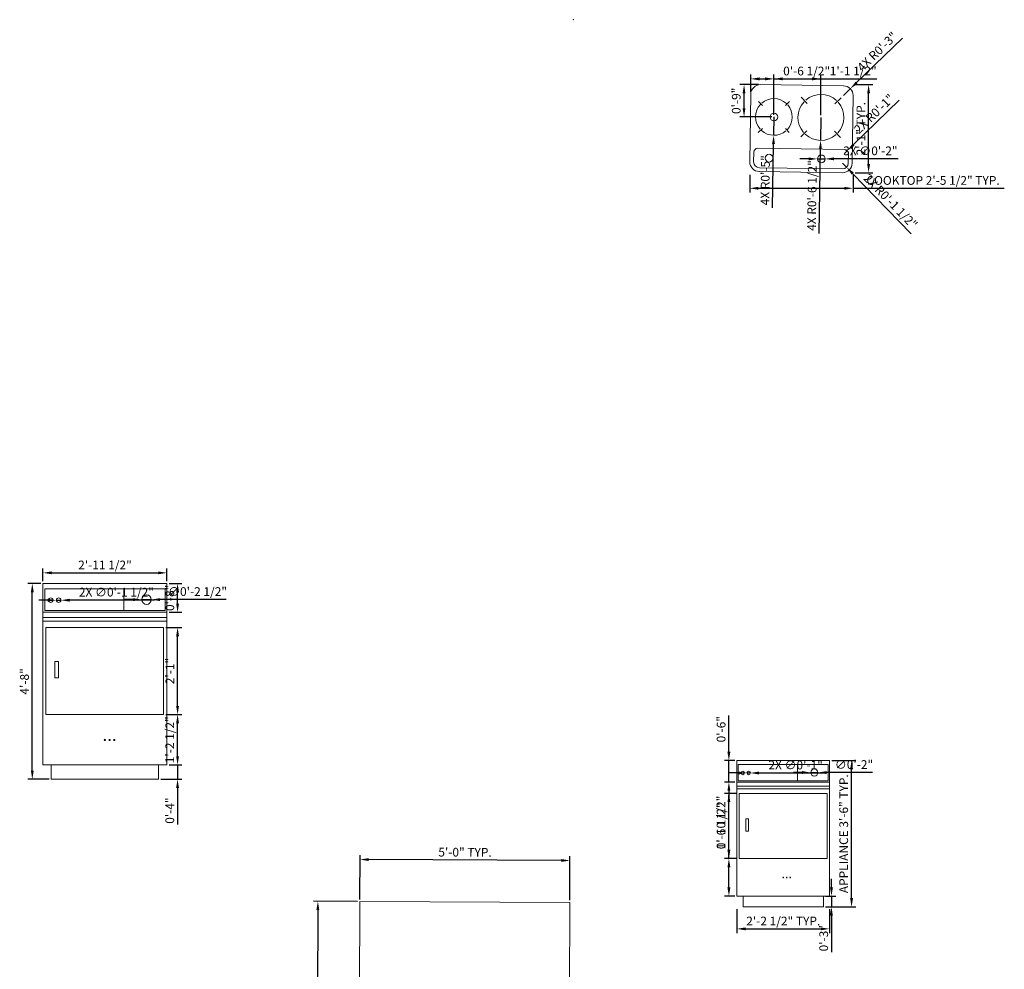
# Model space of a CAD drawing. Units: inches. Extents: x -2945 to -2182, y 3541 to 4172.
# Tile 2 of 5: x -2856 to -2574, y 3900 to 4172. Entities that reach past the tile are written whole.
import ezdxf
from ezdxf.enums import TextEntityAlignment as Align

# ---------------------------------------------------------------- set-up
doc = ezdxf.new("R2010")
doc.units = ezdxf.units.IN
for name, color, linetype, lineweight in [('A-ANNO-DIMS', 2, 'Continuous', 18), ('A-EQPM', 8, 'Continuous', 18), ('A-FURN', 9, 'Continuous', 18), ('A-REFR', 8, 'Continuous', 13)]:
    doc.layers.add(name, color=color, linetype=linetype, lineweight=lineweight)
doc.layers.add('OP-TXT-N2', color=3, linetype='Continuous')
doc.styles.add('OPUS', font='txt')
doc.styles.get("Standard").update_dxf_attribs({"font": 'arial.ttf'})
doc.dimstyles.new('ISO-25', dxfattribs={"dimtxt": 2.5, "dimasz": 2.5, "dimexe": 1.25, "dimexo": 0.625, "dimtad": 1, "dimdec": 0, "dimlunit": 3, "dimtxsty": 'Standard', "dimcen": 2.5, "dimadec": 0, "dimazin": 0, "dimtfac": 1, "dimtdec": 0, "dimtmove": 0, "dimatfit": 3, "dimfxl": 1, "dimarcsym": 0})

# ---------------------------------------------------------------- blocks, each defined once
blk = doc.blocks.new('Bed - Queen')
for p, q in [((0, -80.00003), (0, 0)), ((0, 0), (59.99999, 0)), ((59.99999, 0), (59.99999, -80.00003)), ((7.99999, -1.2), (28.79998, -1.2)), ((7.99999, -14.4), (7.99999, -1.2)), ((28.79998, -1.2), (28.79998, -14.4)), ((31.19999, -1.2), (51.99999, -1.2)), ((31.19999, -14.4), (31.19999, -1.2)), ((51.99999, -1.2), (51.99999, -16.4)), ((0, -14.4), (44.8, -14.4)), ((44.8, -16.8), (0, -16.8)), ((59.99999, -29.6), (44.8, -14.4)), ((44.8, -14.4), (44.8, -29.6)), ((51.99999, -16.4), (46.79936, -16.4)), ((44.8, -29.6), (59.99999, -29.6)), ((59.99999, -80.00003), (0, -80.00003))]:
    blk.add_line(p, q)
blk = doc.blocks.new('COOKTOP-2B')
for p, q in [((26.79, 24.83), (3.07, 25.16)), ((0.27, 22.44), (0, 3.13)), ((2.48, 20.39), (3.6, 19.22)), ((11.35, 20.32), (10.18, 19.2)), ((14.72, 21.57), (16.43, 19.81)), ((26.08, 21.42), (24.32, 19.71)), ((29.25, 2.72), (29.51, 22.03)), ((2.41, 11.52), (3.59, 12.64)), ((11.28, 11.45), (10.16, 12.63)), ((14.56, 10.21), (16.33, 11.92)), ((25.93, 10.06), (24.22, 11.82)), ((1.14, 5.87), (1.1, 3.11)), ((27.09, 6.61), (2.26, 6.96)), ((28.14, 2.74), (28.18, 5.5)), ((2.72, 0.33), (26.45, 0)), ((2.74, 1.43), (26.46, 1.1))]:
    blk.add_line(p, q)
for centre in [(6.88, 15.92), (5.53, 4.15), (20.43, 3.95)]:
    blk.add_circle(centre, 1.1)
for centre, radius, start, end in [((3.03, 22.4), 2.76, 89.203, 179.203), ((26.76, 22.07), 2.76, 359.203, 89.203), ((6.88, 15.92), 5.24, 47.22, 131.186), ((20.32, 15.81), 6.57, 137.22, 221.186), ((20.32, 15.81), 6.57, 47.22, 131.186), ((20.32, 15.81), 6.57, 317.22, 41.186), ((6.88, 15.92), 5.24, 137.22, 221.186), ((6.88, 15.92), 5.24, 317.22, 41.186), ((6.88, 15.92), 5.24, 227.22, 311.186), ((20.32, 15.81), 6.57, 227.22, 311.186), ((2.25, 5.86), 1.1, 89.203, 179.203), ((27.08, 5.51), 1.1, 359.203, 89.203), ((2.76, 3.09), 2.76, 179.203, 269.203), ((2.76, 3.09), 1.66, 179.203, 269.203), ((26.49, 2.76), 2.76, 269.203, 359.203), ((26.49, 2.76), 1.66, 269.203, 359.203)]:
    blk.add_arc(centre, radius, start, end)
blk = doc.blocks.new('KITCHEN-APPLIANCE-FRONT')
for p, q in [((0, 41.84), (0, 3.07)), ((0, 41.84), (26.49, 41.84)), ((0.38, 40.69), (0.38, 36.08)), ((0.38, 40.69), (26.1, 40.69)), ((17.27, 40.69), (17.27, 36.08)), ((26.1, 40.69), (26.1, 36.08)), ((26.49, 41.84), (26.49, 3.07)), ((0, 35.7), (26.49, 35.7)), ((0, 34.55), (26.49, 34.55)), ((0, 33.78), (26.49, 33.78)), ((0.38, 36.08), (26.1, 36.08)), ((0, 3.07), (26.49, 3.07)), ((1.77, 3.07), (1.77, 0)), ((24.72, 3.07), (24.72, 0)), ((24.72, 0), (1.77, 0))]:
    blk.add_line(p, q)
for points in [[(0.62, 13.82), (25.76, 13.82), (25.76, 32.44), (0.62, 32.44)], [(2.53, 21.69), (2.53, 25.14), (3.3, 25.14), (3.3, 21.69)]]:
    blk.add_lwpolyline(points, close=True)
for centre, radius in [((22.13, 38.4), 1.02), ((1.65, 38.28), 0.491), ((3.34, 38.28), 0.491)]:
    blk.add_circle(centre, radius)
at = {"style": 'OPUS'}
blk.add_text('...', height=2.65, dxfattribs=at).set_placement((14.24, 8.2), align=Align.CENTER)
blk = doc.blocks.new('*D12')
at = {"layer": 'A-ANNO-DIMS', "color": 0, "lineweight": -2, "transparency": 16777216}
for p, q in [((-2759.27, 3919.61), (-2771.89, 3919.67)), ((-2770.65, 3917.16), (-2770.99, 3842.16)), ((-2759.63, 3839.61), (-2772.25, 3839.67))]:
    blk.add_line(p, q, dxfattribs=at)
at = {"layer": 'A-ANNO-DIMS', "color": 0, "transparency": 16777216}
for points in [[(-2771.07, 3917.16), (-2770.23, 3917.16), (-2770.64, 3919.66)], [(-2771.41, 3842.16), (-2770.58, 3842.16), (-2771, 3839.66)]]:
    blk.add_solid(points, dxfattribs=at)
at = {"layer": 'Defpoints', "color": 0, "transparency": 16777216}
for p in [(-2758.64, 3919.61), (-2771, 3839.66), (-2759, 3839.61)]:
    blk.add_point(p, dxfattribs=at)
at = {"layer": 'A-ANNO-DIMS', "color": 0, "transparency": 16777216, "insert": (-2772.82, 3879.67), "char_height": 2.5, "attachment_point": 5, "rotation": 89.7398}
blk.add_mtext('QUEEN BED 6\'-8" TYP.', dxfattribs=at)
blk = doc.blocks.new('*D13')
at = {"layer": 'A-ANNO-DIMS', "color": 0, "lineweight": -2, "transparency": 16777216}
for p, q in [((-2758.64, 3920.23), (-2758.58, 3932.86)), ((-2698.64, 3919.96), (-2698.58, 3932.58)), ((-2701.09, 3931.34), (-2756.09, 3931.59))]:
    blk.add_line(p, q, dxfattribs=at)
at = {"layer": 'A-ANNO-DIMS', "color": 0, "transparency": 16777216}
for points in [[(-2756.08, 3932.01), (-2756.09, 3931.18), (-2758.59, 3931.61)], [(-2701.08, 3931.76), (-2701.09, 3930.93), (-2698.59, 3931.33)]]:
    blk.add_solid(points, dxfattribs=at)
at = {"layer": 'Defpoints', "color": 0, "transparency": 16777216}
for p in [(-2758.59, 3931.61), (-2758.64, 3919.61), (-2698.64, 3919.33)]:
    blk.add_point(p, dxfattribs=at)
at = {"layer": 'A-ANNO-DIMS', "color": 0, "transparency": 16777216, "insert": (-2728.58, 3933.37), "char_height": 2.5, "attachment_point": 5, "rotation": 359.7398}
blk.add_mtext('5\'-0" TYP.', dxfattribs=at)
blk = doc.blocks.new('*D14')
at = {"layer": 'A-ANNO-DIMS', "color": 0, "lineweight": -2, "transparency": 16777216}
for p, q in [((-2647.2, 4127.28), (-2647.2, 4122.22)), ((-2617.66, 4127.28), (-2617.66, 4122.22)), ((-2644.7, 4123.47), (-2620.16, 4123.47)), ((-2617.66, 4123.47), (-2574.44, 4123.47))]:
    blk.add_line(p, q, dxfattribs=at)
at = {"layer": 'A-ANNO-DIMS', "color": 0, "transparency": 16777216}
for points in [[(-2644.7, 4123.89), (-2644.7, 4123.06), (-2647.2, 4123.47)], [(-2620.16, 4123.89), (-2620.16, 4123.06), (-2617.66, 4123.47)]]:
    blk.add_solid(points, dxfattribs=at)
at = {"layer": 'Defpoints', "color": 0, "transparency": 16777216}
for p in [(-2647.2, 4127.91), (-2617.66, 4127.91), (-2617.66, 4123.47)]:
    blk.add_point(p, dxfattribs=at)
at = {"layer": 'A-ANNO-DIMS', "color": 0, "transparency": 16777216, "insert": (-2594.8, 4125.39), "char_height": 2.5, "attachment_point": 5}
blk.add_mtext('COOKTOP 2\'-5 1/2" TYP.', dxfattribs=at)
blk = doc.blocks.new('*D15')
at = {"layer": 'A-ANNO-DIMS', "color": 0, "lineweight": -2, "transparency": 16777216}
for p, q in [((-2617.03, 4153.11), (-2611.98, 4153.11)), ((-2613.23, 4130.41), (-2613.23, 4150.61)), ((-2617.03, 4127.91), (-2611.98, 4127.91))]:
    blk.add_line(p, q, dxfattribs=at)
at = {"layer": 'A-ANNO-DIMS', "color": 0, "transparency": 16777216}
for points in [[(-2613.64, 4150.61), (-2612.81, 4150.61), (-2613.23, 4153.11)], [(-2613.64, 4130.41), (-2612.81, 4130.41), (-2613.23, 4127.91)]]:
    blk.add_solid(points, dxfattribs=at)
at = {"layer": 'Defpoints', "color": 0, "transparency": 16777216}
for p in [(-2617.66, 4153.11), (-2613.23, 4153.11), (-2617.66, 4127.91)]:
    blk.add_point(p, dxfattribs=at)
at = {"layer": 'A-ANNO-DIMS', "color": 0, "transparency": 16777216, "insert": (-2615.11, 4140.51), "char_height": 2.5, "attachment_point": 5, "rotation": 90}
blk.add_mtext('2\'-1" TYP.', dxfattribs=at)
blk = doc.blocks.new('*D16')
at = {"layer": 'A-ANNO-DIMS', "color": 0, "lineweight": -2, "transparency": 16777216}
for p, q in [((-2623.75, 3959.91), (-2616.85, 3959.91)), ((-2618.1, 3920.57), (-2618.1, 3957.41)), ((-2623.75, 3918.07), (-2616.85, 3918.07))]:
    blk.add_line(p, q, dxfattribs=at)
at = {"layer": 'A-ANNO-DIMS', "color": 0, "transparency": 16777216}
for points in [[(-2618.51, 3957.41), (-2617.68, 3957.41), (-2618.1, 3959.91)], [(-2618.51, 3920.57), (-2617.68, 3920.57), (-2618.1, 3918.07)]]:
    blk.add_solid(points, dxfattribs=at)
at = {"layer": 'Defpoints', "color": 0, "transparency": 16777216}
for p in [(-2624.37, 3959.91), (-2618.1, 3959.91), (-2624.37, 3918.07)]:
    blk.add_point(p, dxfattribs=at)
at = {"layer": 'A-ANNO-DIMS', "color": 0, "transparency": 16777216, "insert": (-2620.02, 3938.99), "char_height": 2.5, "attachment_point": 5, "rotation": 90}
blk.add_mtext('APPLIANCE 3\'-6" TYP.', dxfattribs=at)
blk = doc.blocks.new('*D17')
at = {"layer": 'A-ANNO-DIMS', "color": 0, "lineweight": -2, "transparency": 16777216}
for p, q in [((-2650.86, 3917.45), (-2650.86, 3910.55)), ((-2624.37, 3917.45), (-2624.37, 3910.55)), ((-2648.36, 3911.8), (-2626.87, 3911.8))]:
    blk.add_line(p, q, dxfattribs=at)
at = {"layer": 'A-ANNO-DIMS', "color": 0, "transparency": 16777216}
for points in [[(-2648.36, 3912.21), (-2648.36, 3911.38), (-2650.86, 3911.8)], [(-2626.87, 3912.21), (-2626.87, 3911.38), (-2624.37, 3911.8)]]:
    blk.add_solid(points, dxfattribs=at)
at = {"layer": 'Defpoints', "color": 0, "transparency": 16777216}
for p in [(-2650.86, 3918.07), (-2624.37, 3918.07), (-2624.37, 3911.8)]:
    blk.add_point(p, dxfattribs=at)
at = {"layer": 'A-ANNO-DIMS', "color": 0, "transparency": 16777216, "insert": (-2637.62, 3913.71), "char_height": 2.5, "attachment_point": 5}
blk.add_mtext('2\'-2 1/2" TYP.', dxfattribs=at)
blk = doc.blocks.new('*D58')
at = {"layer": 'A-ANNO-DIMS', "color": 0, "lineweight": -2, "transparency": 16777216}
for p, q in [((-2849.22, 4011.13), (-2849.22, 4014.8)), ((-2846.72, 4013.55), (-2816.29, 4013.55)), ((-2813.79, 4011.13), (-2813.79, 4014.8))]:
    blk.add_line(p, q, dxfattribs=at)
at = {"layer": 'A-ANNO-DIMS', "color": 0, "transparency": 16777216}
for points in [[(-2846.72, 4013.97), (-2846.72, 4013.14), (-2849.22, 4013.55)], [(-2816.29, 4013.97), (-2816.29, 4013.14), (-2813.79, 4013.55)]]:
    blk.add_solid(points, dxfattribs=at)
at = {"layer": 'Defpoints', "color": 0, "transparency": 16777216}
for p in [(-2813.79, 4013.55), (-2849.22, 4010.5), (-2813.79, 4010.5)]:
    blk.add_point(p, dxfattribs=at)
at = {"layer": 'A-ANNO-DIMS', "color": 0, "transparency": 16777216, "insert": (-2831.5, 4015.47), "char_height": 2.5, "attachment_point": 5}
blk.add_mtext('2\'-11 1/2"', dxfattribs=at)
blk = doc.blocks.new('*D59')
at = {"layer": 'A-ANNO-DIMS', "color": 0, "lineweight": -2, "transparency": 16777216}
for p, q in [((-2849.84, 4010.5), (-2853.52, 4010.5)), ((-2852.27, 3957.04), (-2852.27, 4008)), ((-2847.48, 3954.54), (-2853.52, 3954.54))]:
    blk.add_line(p, q, dxfattribs=at)
at = {"layer": 'A-ANNO-DIMS', "color": 0, "transparency": 16777216}
for points in [[(-2852.68, 4008), (-2851.85, 4008), (-2852.27, 4010.5)], [(-2852.68, 3957.04), (-2851.85, 3957.04), (-2852.27, 3954.54)]]:
    blk.add_solid(points, dxfattribs=at)
at = {"layer": 'Defpoints', "color": 0, "transparency": 16777216}
for p in [(-2852.27, 4010.5), (-2849.22, 4010.5), (-2846.85, 3954.54)]:
    blk.add_point(p, dxfattribs=at)
at = {"layer": 'A-ANNO-DIMS', "color": 0, "transparency": 16777216, "insert": (-2854.17, 3982.52), "char_height": 2.5, "attachment_point": 5, "rotation": 90}
blk.add_mtext('4\'-8"', dxfattribs=at)
blk = doc.blocks.new('*D60')
at = {"layer": 'A-ANNO-DIMS', "color": 0, "lineweight": -2, "transparency": 16777216}
for p, q in [((-2814.14, 3997.93), (-2809.49, 3997.93)), ((-2810.74, 3975.53), (-2810.74, 3995.43)), ((-2814.14, 3973.03), (-2809.49, 3973.03))]:
    blk.add_line(p, q, dxfattribs=at)
at = {"layer": 'A-ANNO-DIMS', "color": 0, "transparency": 16777216}
for points in [[(-2811.16, 3995.43), (-2810.33, 3995.43), (-2810.74, 3997.93)], [(-2811.16, 3975.53), (-2810.33, 3975.53), (-2810.74, 3973.03)]]:
    blk.add_solid(points, dxfattribs=at)
at = {"layer": 'Defpoints', "color": 0, "transparency": 16777216}
for p in [(-2814.77, 3997.93), (-2810.74, 3997.93), (-2814.77, 3973.03)]:
    blk.add_point(p, dxfattribs=at)
at = {"layer": 'A-ANNO-DIMS', "color": 0, "transparency": 16777216, "insert": (-2812.62, 3985.48), "char_height": 2.5, "attachment_point": 5, "rotation": 90}
blk.add_mtext('2\'-1"', dxfattribs=at)
blk = doc.blocks.new('*D61')
at = {"layer": 'A-ANNO-DIMS', "color": 0, "lineweight": -2, "transparency": 16777216}
for p, q in [((-2813.17, 4010.5), (-2809.49, 4010.5)), ((-2810.74, 4004.79), (-2810.74, 4008)), ((-2813.17, 4002.29), (-2809.49, 4002.29))]:
    blk.add_line(p, q, dxfattribs=at)
at = {"layer": 'A-ANNO-DIMS', "color": 0, "transparency": 16777216}
for points in [[(-2811.16, 4008), (-2810.33, 4008), (-2810.74, 4010.5)], [(-2811.16, 4004.79), (-2810.33, 4004.79), (-2810.74, 4002.29)]]:
    blk.add_solid(points, dxfattribs=at)
at = {"layer": 'Defpoints', "color": 0, "transparency": 16777216}
for p in [(-2813.79, 4010.5), (-2810.74, 4010.5), (-2813.79, 4002.29)]:
    blk.add_point(p, dxfattribs=at)
at = {"layer": 'A-ANNO-DIMS', "color": 0, "transparency": 16777216, "insert": (-2812.64, 4006.4), "char_height": 2.5, "attachment_point": 5, "rotation": 90}
blk.add_mtext('0\'-8"', dxfattribs=at)
blk = doc.blocks.new('*D62')
at = {"layer": 'A-ANNO-DIMS', "color": 0, "lineweight": -2, "transparency": 16777216}
for p, q in [((-2810.74, 3961.15), (-2810.74, 3963.65)), ((-2813.17, 3958.65), (-2809.49, 3958.65)), ((-2810.74, 3958.65), (-2810.74, 3954.54)), ((-2815.53, 3954.54), (-2809.49, 3954.54)), ((-2810.74, 3952.04), (-2810.74, 3941.65))]:
    blk.add_line(p, q, dxfattribs=at)
at = {"layer": 'A-ANNO-DIMS', "color": 0, "transparency": 16777216}
for points in [[(-2811.16, 3961.15), (-2810.33, 3961.15), (-2810.74, 3958.65)], [(-2811.16, 3952.04), (-2810.33, 3952.04), (-2810.74, 3954.54)]]:
    blk.add_solid(points, dxfattribs=at)
at = {"layer": 'Defpoints', "color": 0, "transparency": 16777216}
for p in [(-2813.79, 3958.65), (-2816.16, 3954.54), (-2810.74, 3954.54)]:
    blk.add_point(p, dxfattribs=at)
at = {"layer": 'A-ANNO-DIMS', "color": 0, "transparency": 16777216, "insert": (-2812.64, 3945.6), "char_height": 2.5, "attachment_point": 5, "rotation": 90}
blk.add_mtext('0\'-4"', dxfattribs=at)
blk = doc.blocks.new('*D63')
at = {"layer": 'A-ANNO-DIMS', "color": 0, "lineweight": -2, "transparency": 16777216}
for p, q in [((-2814.14, 3973.03), (-2809.49, 3973.03)), ((-2810.74, 3961.15), (-2810.74, 3970.53)), ((-2813.17, 3958.65), (-2809.49, 3958.65))]:
    blk.add_line(p, q, dxfattribs=at)
at = {"layer": 'A-ANNO-DIMS', "color": 0, "transparency": 16777216}
for points in [[(-2811.16, 3970.53), (-2810.33, 3970.53), (-2810.74, 3973.03)], [(-2811.16, 3961.15), (-2810.33, 3961.15), (-2810.74, 3958.65)]]:
    blk.add_solid(points, dxfattribs=at)
at = {"layer": 'Defpoints', "color": 0, "transparency": 16777216}
for p in [(-2814.77, 3973.03), (-2810.74, 3973.03), (-2813.79, 3958.65)]:
    blk.add_point(p, dxfattribs=at)
at = {"layer": 'A-ANNO-DIMS', "color": 0, "transparency": 16777216, "insert": (-2812.66, 3965.84), "char_height": 2.5, "attachment_point": 5, "rotation": 90}
blk.add_mtext('1\'-2 1/2"', dxfattribs=at)
blk = doc.blocks.new('*D64')
at = {"layer": 'A-ANNO-DIMS', "color": 0, "lineweight": -2, "transparency": 16777216}
for p, q in [((-2640.3, 4144.47), (-2640.3, 4155.99)), ((-2637.8, 4154.74), (-2629.36, 4154.74)), ((-2626.86, 4144.37), (-2626.86, 4155.99)), ((-2626.86, 4154.74), (-2610.88, 4154.74))]:
    blk.add_line(p, q, dxfattribs=at)
at = {"layer": 'A-ANNO-DIMS', "color": 0, "transparency": 16777216}
for points in [[(-2637.8, 4155.16), (-2637.8, 4154.32), (-2640.3, 4154.74)], [(-2629.36, 4155.16), (-2629.36, 4154.32), (-2626.86, 4154.74)]]:
    blk.add_solid(points, dxfattribs=at)
at = {"layer": 'Defpoints', "color": 0, "transparency": 16777216}
for p in [(-2626.86, 4154.74), (-2640.3, 4143.85), (-2626.86, 4143.74)]:
    blk.add_point(p, dxfattribs=at)
at = {"layer": 'A-ANNO-DIMS', "color": 0, "transparency": 16777216, "insert": (-2617.62, 4156.66), "char_height": 2.5, "attachment_point": 5}
blk.add_mtext('1\'-1 1/2"', dxfattribs=at)
blk = doc.blocks.new('*D65')
at = {"layer": 'A-ANNO-DIMS', "color": 0, "lineweight": -2, "transparency": 16777216}
for p, q in [((-2644.74, 4153.09), (-2650.08, 4153.09)), ((-2648.83, 4146.35), (-2648.83, 4150.59)), ((-2640.93, 4143.85), (-2650.08, 4143.85))]:
    blk.add_line(p, q, dxfattribs=at)
at = {"layer": 'A-ANNO-DIMS', "color": 0, "transparency": 16777216}
for points in [[(-2649.25, 4150.59), (-2648.42, 4150.59), (-2648.83, 4153.09)], [(-2649.25, 4146.35), (-2648.42, 4146.35), (-2648.83, 4143.85)]]:
    blk.add_solid(points, dxfattribs=at)
at = {"layer": 'Defpoints', "color": 0, "transparency": 16777216}
for p in [(-2648.83, 4153.09), (-2644.12, 4153.09), (-2640.3, 4143.85)]:
    blk.add_point(p, dxfattribs=at)
at = {"layer": 'A-ANNO-DIMS', "color": 0, "transparency": 16777216, "insert": (-2650.73, 4148.47), "char_height": 2.5, "attachment_point": 5, "rotation": 90}
blk.add_mtext('0\'-9"', dxfattribs=at)
blk = doc.blocks.new('*D66')
at = {"layer": 'A-ANNO-DIMS', "color": 0, "lineweight": -2, "transparency": 16777216}
for p, q in [((-2646.91, 4150.99), (-2646.91, 4155.99)), ((-2644.41, 4154.74), (-2642.8, 4154.74)), ((-2640.3, 4144.47), (-2640.3, 4155.99)), ((-2640.3, 4154.74), (-2624.08, 4154.74))]:
    blk.add_line(p, q, dxfattribs=at)
at = {"layer": 'A-ANNO-DIMS', "color": 0, "transparency": 16777216}
for points in [[(-2644.41, 4155.16), (-2644.41, 4154.32), (-2646.91, 4154.74)], [(-2642.8, 4155.16), (-2642.8, 4154.32), (-2640.3, 4154.74)]]:
    blk.add_solid(points, dxfattribs=at)
at = {"layer": 'Defpoints', "color": 0, "transparency": 16777216}
for p in [(-2640.3, 4154.74), (-2646.91, 4150.37), (-2640.3, 4143.85)]:
    blk.add_point(p, dxfattribs=at)
at = {"layer": 'A-ANNO-DIMS', "color": 0, "transparency": 16777216, "insert": (-2630.94, 4156.66), "char_height": 2.5, "attachment_point": 5}
blk.add_mtext('0\'-6 1/2"', dxfattribs=at)
blk = doc.blocks.new('*D67')
at = {"layer": 'A-ANNO-DIMS', "color": 0, "lineweight": -2, "transparency": 16777216}
for p, q in [((-2653.16, 3931.89), (-2653.16, 3950.05)), ((-2650.87, 3931.89), (-2654.41, 3931.89)), ((-2653.16, 3923.64), (-2653.16, 3929.39)), ((-2651.49, 3921.14), (-2654.41, 3921.14))]:
    blk.add_line(p, q, dxfattribs=at)
at = {"layer": 'A-ANNO-DIMS', "color": 0, "transparency": 16777216}
for points in [[(-2653.58, 3929.39), (-2652.74, 3929.39), (-2653.16, 3931.89)], [(-2653.58, 3923.64), (-2652.74, 3923.64), (-2653.16, 3921.14)]]:
    blk.add_solid(points, dxfattribs=at)
at = {"layer": 'Defpoints', "color": 0, "transparency": 16777216}
for p in [(-2653.16, 3931.89), (-2650.25, 3931.89), (-2650.86, 3921.14)]:
    blk.add_point(p, dxfattribs=at)
at = {"layer": 'A-ANNO-DIMS', "color": 0, "transparency": 16777216, "insert": (-2655.08, 3942.22), "char_height": 2.5, "attachment_point": 5, "rotation": 90}
blk.add_mtext('0\'-10 1/2"', dxfattribs=at)
blk = doc.blocks.new('*D68')
at = {"layer": 'A-ANNO-DIMS', "color": 0, "lineweight": -2, "transparency": 16777216}
for p, q in [((-2650.87, 3950.51), (-2654.41, 3950.51)), ((-2653.16, 3934.39), (-2653.16, 3948.01)), ((-2650.87, 3931.89), (-2654.41, 3931.89))]:
    blk.add_line(p, q, dxfattribs=at)
at = {"layer": 'A-ANNO-DIMS', "color": 0, "transparency": 16777216}
for points in [[(-2653.58, 3948.01), (-2652.74, 3948.01), (-2653.16, 3950.51)], [(-2653.58, 3934.39), (-2652.74, 3934.39), (-2653.16, 3931.89)]]:
    blk.add_solid(points, dxfattribs=at)
at = {"layer": 'Defpoints', "color": 0, "transparency": 16777216}
for p in [(-2653.16, 3950.51), (-2650.25, 3950.51), (-2650.25, 3931.89)]:
    blk.add_point(p, dxfattribs=at)
at = {"layer": 'A-ANNO-DIMS', "color": 0, "transparency": 16777216, "insert": (-2655.08, 3941.2), "char_height": 2.5, "attachment_point": 5, "rotation": 90}
blk.add_mtext('1\'-6 1/2"', dxfattribs=at)
blk = doc.blocks.new('*D69')
at = {"layer": 'A-ANNO-DIMS', "color": 0, "lineweight": -2, "transparency": 16777216}
for p, q in [((-2653.16, 3962.41), (-2653.16, 3972.81)), ((-2651.49, 3959.91), (-2654.41, 3959.91)), ((-2653.16, 3953.77), (-2653.16, 3959.91)), ((-2651.49, 3953.77), (-2654.41, 3953.77)), ((-2653.16, 3951.27), (-2653.16, 3948.77))]:
    blk.add_line(p, q, dxfattribs=at)
at = {"layer": 'A-ANNO-DIMS', "color": 0, "transparency": 16777216}
for points in [[(-2653.58, 3962.41), (-2652.74, 3962.41), (-2653.16, 3959.91)], [(-2653.58, 3951.27), (-2652.74, 3951.27), (-2653.16, 3953.77)]]:
    blk.add_solid(points, dxfattribs=at)
at = {"layer": 'Defpoints', "color": 0, "transparency": 16777216}
for p in [(-2653.16, 3959.91), (-2650.86, 3959.91), (-2650.86, 3953.77)]:
    blk.add_point(p, dxfattribs=at)
at = {"layer": 'A-ANNO-DIMS', "color": 0, "transparency": 16777216, "insert": (-2655.06, 3968.86), "char_height": 2.5, "attachment_point": 5, "rotation": 90}
blk.add_mtext('0\'-6"', dxfattribs=at)
blk = doc.blocks.new('*D70')
at = {"layer": 'A-ANNO-DIMS', "color": 0, "lineweight": -2, "transparency": 16777216}
for p, q in [((-2623.84, 3923.64), (-2623.84, 3926.14)), ((-2625.52, 3921.14), (-2622.59, 3921.14)), ((-2623.84, 3921.14), (-2623.84, 3918.07)), ((-2625.52, 3918.07), (-2622.59, 3918.07)), ((-2623.84, 3915.57), (-2623.84, 3905.18))]:
    blk.add_line(p, q, dxfattribs=at)
at = {"layer": 'A-ANNO-DIMS', "color": 0, "transparency": 16777216}
for points in [[(-2624.26, 3923.64), (-2623.43, 3923.64), (-2623.84, 3921.14)], [(-2624.26, 3915.57), (-2623.43, 3915.57), (-2623.84, 3918.07)]]:
    blk.add_solid(points, dxfattribs=at)
at = {"layer": 'Defpoints', "color": 0, "transparency": 16777216}
for p in [(-2626.14, 3921.14), (-2626.14, 3918.07), (-2623.84, 3918.07)]:
    blk.add_point(p, dxfattribs=at)
at = {"layer": 'A-ANNO-DIMS', "color": 0, "transparency": 16777216, "insert": (-2625.74, 3909.12), "char_height": 2.5, "attachment_point": 5, "rotation": 90}
blk.add_mtext('0\'-3"', dxfattribs=at)
blk = doc.blocks.new('*D78')
at = {"layer": 'A-ANNO-DIMS', "color": 0, "lineweight": -2, "transparency": 16777216}
for p, q in [((-2823.47, 4005.9), (-2825.97, 4005.9)), ((-2820.97, 4005.9), (-2818.25, 4005.9)), ((-2796.81, 4005.89), (-2815.75, 4005.9))]:
    blk.add_line(p, q, dxfattribs=at)
at = {"layer": 'A-ANNO-DIMS', "color": 0, "transparency": 16777216}
for points in [[(-2823.47, 4006.32), (-2823.47, 4005.48), (-2820.97, 4005.9)], [(-2815.75, 4006.31), (-2815.75, 4005.48), (-2818.25, 4005.9)]]:
    blk.add_solid(points, dxfattribs=at)
at = {"layer": 'Defpoints', "color": 0, "transparency": 16777216}
for p in [(-2820.97, 4005.9), (-2818.25, 4005.9)]:
    blk.add_point(p, dxfattribs=at)
at = {"layer": 'A-ANNO-DIMS', "color": 0, "transparency": 16777216, "insert": (-2805.03, 4007.87), "char_height": 2.5, "attachment_point": 5, "rotation": 359.9815}
blk.add_mtext('∅0\'-2 1/2"', dxfattribs=at)
blk = doc.blocks.new('*D79')
at = {"layer": 'A-ANNO-DIMS', "color": 0, "lineweight": -2, "transparency": 16777216}
for p, q in [((-2847.9, 4005.73), (-2850.4, 4005.73)), ((-2845.4, 4005.73), (-2844.09, 4005.73)), ((-2817.37, 4005.75), (-2841.59, 4005.74))]:
    blk.add_line(p, q, dxfattribs=at)
at = {"layer": 'A-ANNO-DIMS', "color": 0, "transparency": 16777216}
for points in [[(-2847.9, 4006.15), (-2847.9, 4005.32), (-2845.4, 4005.73)], [(-2841.59, 4006.15), (-2841.59, 4005.32), (-2844.09, 4005.73)]]:
    blk.add_solid(points, dxfattribs=at)
at = {"layer": 'Defpoints', "color": 0, "transparency": 16777216}
for p in [(-2845.4, 4005.73), (-2844.09, 4005.73)]:
    blk.add_point(p, dxfattribs=at)
at = {"layer": 'A-ANNO-DIMS', "color": 0, "transparency": 16777216, "insert": (-2828.23, 4007.71), "char_height": 2.5, "attachment_point": 5, "rotation": 0.0269}
blk.add_mtext('2X ∅0\'-1 1/2"', dxfattribs=at)
blk = doc.blocks.new('*D80')
at = {"layer": 'A-ANNO-DIMS', "color": 0, "lineweight": -2, "transparency": 16777216}
for p, q in [((-2626.86, 4143.74), (-2626.95, 4137.17)), ((-2627.32, 4110.58), (-2626.99, 4134.67))]:
    blk.add_line(p, q, dxfattribs=at)
at = {"layer": 'A-ANNO-DIMS', "color": 0, "transparency": 16777216}
blk.add_solid([(-2627.4, 4134.67), (-2626.57, 4134.66), (-2626.95, 4137.17)], dxfattribs=at)
at = {"layer": 'Defpoints', "color": 0, "transparency": 16777216}
for p in [(-2626.86, 4143.74), (-2626.95, 4137.17)]:
    blk.add_point(p, dxfattribs=at)
at = {"layer": 'A-ANNO-DIMS', "color": 0, "transparency": 16777216, "insert": (-2629.09, 4121.4), "char_height": 2.5, "attachment_point": 5, "rotation": 89.1998}
blk.add_mtext('4X R0\'-6 1/2"', dxfattribs=at)
blk = doc.blocks.new('*D81')
at = {"layer": 'A-ANNO-DIMS', "color": 0, "lineweight": -2, "transparency": 16777216}
for p, q in [((-2640.3, 4143.85), (-2640.37, 4138.61)), ((-2640.66, 4117.85), (-2640.41, 4136.11))]:
    blk.add_line(p, q, dxfattribs=at)
at = {"layer": 'A-ANNO-DIMS', "color": 0, "transparency": 16777216}
blk.add_solid([(-2640.83, 4136.11), (-2639.99, 4136.1), (-2640.37, 4138.61)], dxfattribs=at)
at = {"layer": 'Defpoints', "color": 0, "transparency": 16777216}
for p in [(-2640.3, 4143.85), (-2640.37, 4138.61)]:
    blk.add_point(p, dxfattribs=at)
at = {"layer": 'A-ANNO-DIMS', "color": 0, "transparency": 16777216, "insert": (-2642.45, 4125.75), "char_height": 2.5, "attachment_point": 5, "rotation": 89.201}
blk.add_mtext('4X R0\'-5"', dxfattribs=at)
blk = doc.blocks.new('*D82')
at = {"layer": 'A-ANNO-DIMS', "color": 0, "lineweight": -2, "transparency": 16777216}
for p, q in [((-2603.57, 4166.4), (-2616.66, 4153.67)), ((-2620.43, 4150), (-2618.45, 4151.92))]:
    blk.add_line(p, q, dxfattribs=at)
at = {"layer": 'A-ANNO-DIMS', "color": 0, "transparency": 16777216}
blk.add_solid([(-2616.95, 4153.96), (-2616.37, 4153.37), (-2618.45, 4151.92)], dxfattribs=at)
at = {"layer": 'Defpoints', "color": 0, "transparency": 16777216}
for p in [(-2618.45, 4151.92), (-2620.43, 4150)]:
    blk.add_point(p, dxfattribs=at)
at = {"layer": 'A-ANNO-DIMS', "color": 0, "transparency": 16777216, "insert": (-2610.54, 4162.27), "char_height": 2.5, "attachment_point": 5, "rotation": 44.1991}
blk.add_mtext('4X R0\'-3"', dxfattribs=at)
blk = doc.blocks.new('*D83')
at = {"layer": 'A-ANNO-DIMS', "color": 0, "lineweight": -2, "transparency": 16777216}
for p, q in [((-2620.7, 4130.69), (-2619.54, 4129.5)), ((-2601.04, 4110.48), (-2617.8, 4127.71))]:
    blk.add_line(p, q, dxfattribs=at)
at = {"layer": 'A-ANNO-DIMS', "color": 0, "transparency": 16777216}
blk.add_solid([(-2617.5, 4128), (-2618.1, 4127.42), (-2619.54, 4129.5)], dxfattribs=at)
at = {"layer": 'Defpoints', "color": 0, "transparency": 16777216}
for p in [(-2620.7, 4130.69), (-2619.54, 4129.5)]:
    blk.add_point(p, dxfattribs=at)
at = {"layer": 'A-ANNO-DIMS', "color": 0, "transparency": 16777216, "insert": (-2607.17, 4119.54), "char_height": 2.5, "attachment_point": 5, "rotation": 314.2095}
blk.add_mtext('2X R0\'-1 1/2"', dxfattribs=at)
blk = doc.blocks.new('*D84')
at = {"layer": 'A-ANNO-DIMS', "color": 0, "lineweight": -2, "transparency": 16777216}
for p, q in [((-2630.35, 4131.87), (-2632.85, 4131.87)), ((-2627.85, 4131.87), (-2625.65, 4131.87)), ((-2604.79, 4131.87), (-2623.15, 4131.87))]:
    blk.add_line(p, q, dxfattribs=at)
at = {"layer": 'A-ANNO-DIMS', "color": 0, "transparency": 16777216}
for points in [[(-2630.35, 4132.29), (-2630.35, 4131.46), (-2627.85, 4131.87)], [(-2623.15, 4132.29), (-2623.15, 4131.46), (-2625.65, 4131.87)]]:
    blk.add_solid(points, dxfattribs=at)
at = {"layer": 'Defpoints', "color": 0, "transparency": 16777216}
for p in [(-2627.85, 4131.87), (-2625.65, 4131.87)]:
    blk.add_point(p, dxfattribs=at)
at = {"layer": 'A-ANNO-DIMS', "color": 0, "transparency": 16777216, "insert": (-2612.72, 4133.84), "char_height": 2.5, "attachment_point": 5, "rotation": 359.994}
blk.add_mtext('3X ∅0\'-2"', dxfattribs=at)
blk = doc.blocks.new('*D85')
at = {"layer": 'A-ANNO-DIMS', "color": 0, "lineweight": -2, "transparency": 16777216}
for p, q in [((-2604.47, 4148.64), (-2617.52, 4135.95)), ((-2620.11, 4133.44), (-2619.31, 4134.21))]:
    blk.add_line(p, q, dxfattribs=at)
at = {"layer": 'A-ANNO-DIMS', "color": 0, "transparency": 16777216}
blk.add_solid([(-2617.81, 4136.25), (-2617.23, 4135.65), (-2619.31, 4134.21)], dxfattribs=at)
at = {"layer": 'Defpoints', "color": 0, "transparency": 16777216}
for p in [(-2620.11, 4133.44), (-2619.31, 4134.21)]:
    blk.add_point(p, dxfattribs=at)
at = {"layer": 'A-ANNO-DIMS', "color": 0, "transparency": 16777216, "insert": (-2611.43, 4144.53), "char_height": 2.5, "attachment_point": 5, "rotation": 44.1933}
blk.add_mtext('2X R0\'-1"', dxfattribs=at)
blk = doc.blocks.new('*D86')
at = {"layer": 'A-ANNO-DIMS', "color": 0, "lineweight": -2, "transparency": 16777216}
for p, q in [((-2632.24, 3956.47), (-2634.74, 3956.47)), ((-2629.74, 3956.47), (-2627.71, 3956.47)), ((-2612.1, 3956.47), (-2625.21, 3956.47))]:
    blk.add_line(p, q, dxfattribs=at)
at = {"layer": 'A-ANNO-DIMS', "color": 0, "transparency": 16777216}
for points in [[(-2632.24, 3956.89), (-2632.24, 3956.06), (-2629.74, 3956.47)], [(-2625.21, 3956.89), (-2625.21, 3956.05), (-2627.71, 3956.47)]]:
    blk.add_solid(points, dxfattribs=at)
at = {"layer": 'Defpoints', "color": 0, "transparency": 16777216}
for p in [(-2629.74, 3956.47), (-2627.71, 3956.47)]:
    blk.add_point(p, dxfattribs=at)
at = {"layer": 'A-ANNO-DIMS', "color": 0, "transparency": 16777216, "insert": (-2617.4, 3958.44), "char_height": 2.5, "attachment_point": 5, "rotation": 359.9785}
blk.add_mtext('∅0\'-2"', dxfattribs=at)
blk = doc.blocks.new('*D87')
at = {"layer": 'A-ANNO-DIMS', "color": 0, "lineweight": -2, "transparency": 16777216}
for p, q in [((-2650.51, 3956.35), (-2653.01, 3956.35)), ((-2648.01, 3956.35), (-2647.03, 3956.35)), ((-2626.13, 3956.33), (-2644.53, 3956.34))]:
    blk.add_line(p, q, dxfattribs=at)
at = {"layer": 'A-ANNO-DIMS', "color": 0, "transparency": 16777216}
for points in [[(-2650.51, 3956.77), (-2650.51, 3955.93), (-2648.01, 3956.35)], [(-2644.53, 3956.76), (-2644.53, 3955.93), (-2647.03, 3956.35)]]:
    blk.add_solid(points, dxfattribs=at)
at = {"layer": 'Defpoints', "color": 0, "transparency": 16777216}
for p in [(-2648.01, 3956.35), (-2647.03, 3956.35)]:
    blk.add_point(p, dxfattribs=at)
at = {"layer": 'A-ANNO-DIMS', "color": 0, "transparency": 16777216, "insert": (-2634.08, 3958.31), "char_height": 2.5, "attachment_point": 5, "rotation": 359.9476}
blk.add_mtext('2X ∅0\'-1"', dxfattribs=at)

msp = doc.modelspace()

# ---------------------------------------------------------------- linework, layer by layer
at = {"layer": 'A-EQPM'}
for p, q in [((-2849.22, 4010.5), (-2849.22, 3958.65)), ((-2849.22, 4010.5), (-2813.79, 4010.5)), ((-2813.79, 4010.5), (-2813.79, 3958.65)), ((-2848.7, 4008.96), (-2848.7, 4002.8)), ((-2848.7, 4008.96), (-2814.31, 4008.96)), ((-2826.11, 4008.96), (-2826.11, 4002.8)), ((-2814.31, 4008.96), (-2814.31, 4002.8)), ((-2849.22, 4002.29), (-2813.79, 4002.29)), ((-2848.7, 4002.8), (-2814.31, 4002.8)), ((-2849.22, 4000.75), (-2813.79, 4000.75)), ((-2849.22, 3999.72), (-2813.79, 3999.72)), ((-2849.22, 3958.65), (-2813.79, 3958.65)), ((-2846.85, 3958.65), (-2846.85, 3954.54)), ((-2816.16, 3958.65), (-2816.16, 3954.54)), ((-2816.16, 3954.54), (-2846.85, 3954.54))]:
    msp.add_line(p, q, dxfattribs=at)
for points in [[(-2848.39, 3973.03), (-2814.77, 3973.03), (-2814.77, 3997.93), (-2848.39, 3997.93)], [(-2845.83, 3983.55), (-2845.83, 3988.17), (-2844.8, 3988.17), (-2844.8, 3983.55)]]:
    msp.add_lwpolyline(points, close=True, dxfattribs=at)
for centre, radius in [((-2847.01, 4005.73), 0.656), ((-2844.74, 4005.73), 0.656), ((-2819.61, 4005.9), 1.36)]:
    msp.add_circle(centre, radius, dxfattribs=at)
at = {"layer": 'A-REFR'}
msp.add_point((-2697.64, 4171.66), dxfattribs=at)

# ---------------------------------------------------------------- block references
at = {"layer": 'A-EQPM'}
for name, p in [('COOKTOP-2B', (-2647.18, 4127.93)), ('KITCHEN-APPLIANCE-FRONT', (-2650.86, 3918.07))]:
    msp.add_blockref(name, p, dxfattribs=at)
at = {"layer": 'A-FURN', "rotation": 179.7397650528711}
msp.add_blockref('Bed - Queen', (-2699, 3839.33), dxfattribs=at)

# ---------------------------------------------------------------- texts
at = {"layer": 'OP-TXT-N2', "style": 'OPUS'}
msp.add_text('...', height=3.544, dxfattribs=at).set_placement((-2830.18, 3965.51), align=Align.CENTER)

# ---------------------------------------------------------------- dimensions: what is measured, and where the dimension line sits
at = {"layer": 'A-ANNO-DIMS'}
for center, mpoint, text, picture, middle in [((-2620.43, 4150), (-2618.45, 4151.92), '4X <>', '*D82', (-2610.54, 4162.27)), ((-2620.11, 4133.44), (-2619.31, 4134.21), '2X <>', '*D85', (-2611.43, 4144.53)), ((-2640.3, 4143.85), (-2640.37, 4138.61), '4X <>', '*D81', (-2642.45, 4125.75)), ((-2626.86, 4143.74), (-2626.95, 4137.17), '4X <>', '*D80', (-2629.09, 4121.4)), ((-2620.7, 4130.69), (-2619.54, 4129.5), '2X <>', '*D83', (-2607.17, 4119.54))]:
    dim = msp.add_radius_dim(center=center, mpoint=mpoint, text=text, dimstyle='ISO-25', override={"dimdec": 1, "dimlfac": 1, "dimrnd": 0, "dimzin": 1, "dimdsep": 46, "dimlunit": 4, "dimfrac": 2}, dxfattribs=at)
    dim.commit()
    dim.dimension.update_dxf_attribs({"geometry": picture, "text_midpoint": middle})
for base, p1, p2, picture, middle in [((-2640.3, 4154.74), (-2646.91, 4150.37), (-2640.3, 4143.85), '*D66', (-2630.94, 4156.66)), ((-2626.86, 4154.74), (-2640.3, 4143.85), (-2626.86, 4143.74), '*D64', (-2617.62, 4156.66)), ((-2813.79, 4013.55), (-2849.22, 4010.5), (-2813.79, 4010.5), '*D58', (-2831.5, 4015.47))]:
    dim = msp.add_linear_dim(base=base, p1=p1, p2=p2, dimstyle='ISO-25', override={"dimdec": 1, "dimlfac": 1, "dimrnd": 0, "dimzin": 1, "dimdsep": 46, "dimlunit": 4, "dimfrac": 2}, dxfattribs=at)
    dim.commit()
    dim.dimension.update_dxf_attribs({"geometry": picture, "text_midpoint": middle})
for base, p1, p2, angle, picture, middle in [((-2648.83, 4153.09), (-2640.3, 4143.85), (-2644.12, 4153.09), 90, '*D65', (-2650.73, 4148.47)), ((-2852.27, 4010.5), (-2846.85, 3954.54), (-2849.22, 4010.5), 90, '*D59', (-2854.17, 3982.52)), ((-2810.74, 4010.5), (-2813.79, 4002.29), (-2813.79, 4010.5), 90, '*D61', (-2812.64, 4006.4)), ((-2810.74, 3997.93), (-2814.77, 3973.03), (-2814.77, 3997.93), 90, '*D60', (-2812.62, 3985.48)), ((-2810.74, 3973.03), (-2813.79, 3958.65), (-2814.77, 3973.03), 90, '*D63', (-2812.66, 3965.84)), ((-2653.16, 3959.91), (-2650.86, 3953.77), (-2650.86, 3959.91), 90, '*D69', (-2655.06, 3968.86)), ((-2810.74, 3954.54), (-2813.79, 3958.65), (-2816.16, 3954.54), 90, '*D62', (-2812.64, 3945.6)), ((-2653.16, 3950.51), (-2650.25, 3931.89), (-2650.25, 3950.51), 90, '*D68', (-2655.08, 3941.2)), ((-2653.1614, 3931.8916), (-2650.8614, 3921.1433), (-2650.2454, 3931.8916), 90, '*D67', (-2655.0791, 3942.2233)), ((-2623.84, 3918.07), (-2626.14, 3921.14), (-2626.14, 3918.07), 270, '*D70', (-2625.74, 3909.12))]:
    dim = msp.add_linear_dim(base=base, p1=p1, p2=p2, angle=angle, dimstyle='ISO-25', override={"dimdec": 1, "dimlfac": 1, "dimrnd": 0, "dimzin": 1, "dimdsep": 46, "dimlunit": 4, "dimfrac": 2}, dxfattribs=at)
    dim.commit()
    dim.dimension.update_dxf_attribs({"geometry": picture, "text_midpoint": middle})
for base, p1, p2, angle, text, picture, middle in [((-2613.23, 4153.11), (-2617.66, 4127.91), (-2617.66, 4153.11), 90, '<> TYP.', '*D15', (-2615.11, 4140.51)), ((-2618.1, 3959.91), (-2624.37, 3918.07), (-2624.37, 3959.91), 90, 'APPLIANCE <> TYP.', '*D16', (-2620.02, 3938.99)), ((-2758.59, 3931.61), (-2698.64, 3919.33), (-2758.64, 3919.61), 179.7398, '<> TYP.', '*D13', (-2728.58, 3933.37)), ((-2771, 3839.66), (-2758.64, 3919.61), (-2759, 3839.61), 269.7398, 'QUEEN BED <> TYP.', '*D12', (-2772.82, 3879.67))]:
    dim = msp.add_linear_dim(base=base, p1=p1, p2=p2, angle=angle, text=text, dimstyle='ISO-25', override={"dimdec": 1, "dimlfac": 1, "dimrnd": 0, "dimzin": 1, "dimdsep": 46, "dimlunit": 4, "dimfrac": 2}, dxfattribs=at)
    dim.commit()
    dim.dimension.update_dxf_attribs({"geometry": picture, "text_midpoint": middle})
for p1, p2, text, picture, middle in [((-2627.85, 4131.87), (-2625.65, 4131.87), '3X <>', '*D84', (-2612.72, 4131.87)), ((-2845.4, 4005.73), (-2844.09, 4005.73), '2X <>', '*D79', (-2828.23, 4005.74))]:
    dim = msp.add_diameter_dim_2p(p1=p1, p2=p2, text=text, dimstyle='ISO-25', override={"dimdec": 1, "dimlfac": 1, "dimrnd": 0, "dimzin": 1, "dimdsep": 46, "dimlunit": 4, "dimfrac": 2}, dxfattribs=at)
    dim.commit()
    dim.dimension.update_dxf_attribs({"geometry": picture, "text_midpoint": middle, "dimtype": 163})
for base, p1, p2, text, picture, middle in [((-2617.66, 4123.47), (-2647.2, 4127.91), (-2617.66, 4127.91), 'COOKTOP <> TYP.', '*D14', (-2594.8, 4125.39)), ((-2624.37, 3911.8), (-2650.86, 3918.07), (-2624.37, 3918.07), '<> TYP.', '*D17', (-2637.62, 3913.71))]:
    dim = msp.add_linear_dim(base=base, p1=p1, p2=p2, text=text, dimstyle='ISO-25', override={"dimdec": 1, "dimlfac": 1, "dimrnd": 0, "dimzin": 1, "dimdsep": 46, "dimlunit": 4, "dimfrac": 2}, dxfattribs=at)
    dim.commit()
    dim.dimension.update_dxf_attribs({"geometry": picture, "text_midpoint": middle})
dim = msp.add_diameter_dim_2p(p1=(-2820.97, 4005.9), p2=(-2818.25, 4005.9), dimstyle='ISO-25', override={"dimdec": 1, "dimlfac": 1, "dimrnd": 0, "dimzin": 1, "dimdsep": 46, "dimlunit": 4, "dimfrac": 2}, dxfattribs=at)
dim.commit()
dim.dimension.update_dxf_attribs({"geometry": '*D78', "text_midpoint": (-2805.03, 4005.89), "dimtype": 163})
dim = msp.add_diameter_dim_2p(p1=(-2648.01, 3956.35), p2=(-2647.03, 3956.35), text='2X <>', dimstyle='ISO-25', override={"dimdec": 1, "dimlfac": 1, "dimrnd": 0, "dimzin": 1, "dimdsep": 46, "dimlunit": 4, "dimfrac": 2}, dxfattribs=at)
dim.commit()
dim.dimension.update_dxf_attribs({"geometry": '*D87', "text_midpoint": (-2634.08, 3956.34)})
dim = msp.add_diameter_dim_2p(p1=(-2629.74, 3956.47), p2=(-2627.71, 3956.47), dimstyle='ISO-25', override={"dimdec": 1, "dimlfac": 1, "dimrnd": 0, "dimzin": 1, "dimdsep": 46, "dimlunit": 4, "dimfrac": 2}, dxfattribs=at)
dim.commit()
dim.dimension.update_dxf_attribs({"geometry": '*D86', "text_midpoint": (-2617.4, 3956.47)})

doc.saveas('drawing.dxf')
